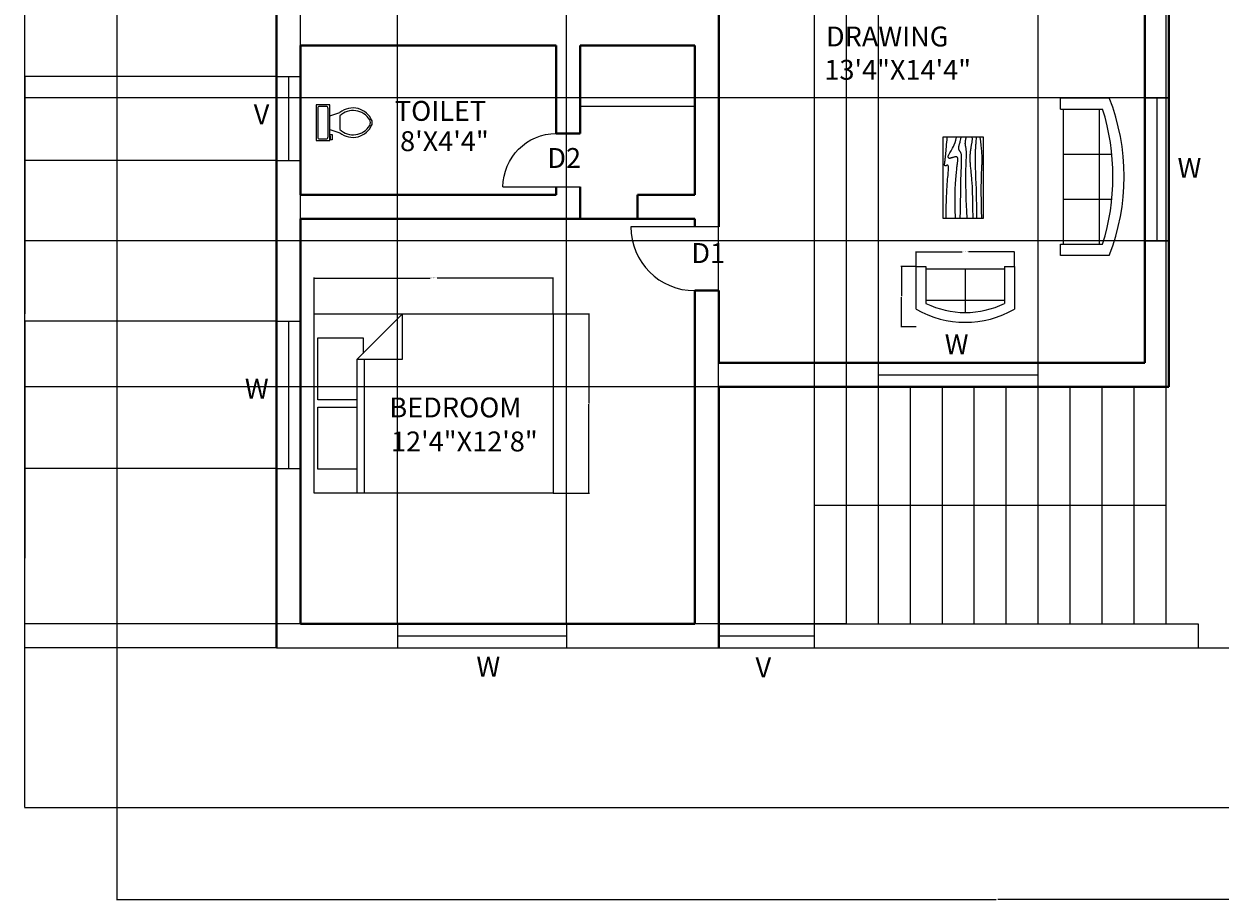
# Model space of a CAD drawing. Units: feet. Extents: x 2032 to 2763, y 1402 to 2145.
# Tile 1 of 6: x 2032 to 2482, y 1402 to 1731. Entities that reach past the tile are written whole.
import ezdxf

# ---------------------------------------------------------------- set-up
doc = ezdxf.new("R2010")
doc.units = ezdxf.units.FT
for name, color, linetype, lineweight in [('A-ANNO-DIMS', 2, 'Continuous', 18), ('A-ANNO-TEXT', 7, 'Continuous', 18), ('A-AREA-IDEN', 7, 'Continuous', 25), ('A-DOOR', 3, 'Continuous', 25), ('A-FLOR', 7, 'Continuous', 25), ('A-FLOR-CASE', 8, 'Continuous', 18), ('A-FLOR-FIXT', 8, 'Continuous', 18), ('A-FLOR-STRS', 7, 'Continuous', 18), ('A-FURN', 8, 'Continuous', 18), ('A-GLAZ', 4, 'Continuous', 18), ('A-WALL', 7, 'Continuous', 40), ('C-PROP', 8, 'Continuous', 25)]:
    doc.layers.add(name, color=color, linetype=linetype, lineweight=lineweight)
doc.styles.get("Standard").update_dxf_attribs({"font": 'arial.ttf'})
doc.dimstyles.get("Standard").update_dxf_attribs({"dimtxt": 0.18, "dimasz": 0.18, "dimexe": 0.18, "dimexo": 0.0625, "dimgap": 0.09, "dimtad": 0, "dimtih": 1, "dimtoh": 1, "dimdec": 4, "dimzin": 0, "dimdsep": 46, "dimtxsty": 'Standard', "dimcen": 0.09, "dimadec": 0, "dimazin": 0, "dimtfac": 1, "dimtdec": 4, "dimtofl": 0, "dimtmove": 0, "dimatfit": 3, "dimfxl": 1, "dimtolj": 1, "dimtzin": 0, "dimarcsym": 0})

# ---------------------------------------------------------------- blocks, each defined once
blk = doc.blocks.new('Bed - Queen')
for p, q in [((0, -80.00003), (0, 0)), ((0, 0), (59.99999, 0)), ((59.99999, 0), (59.99999, -80.00003)), ((7.99999, -1.2), (28.79998, -1.2)), ((7.99999, -14.4), (7.99999, -1.2)), ((28.79998, -1.2), (28.79998, -14.4)), ((31.19999, -1.2), (51.99999, -1.2)), ((31.19999, -14.4), (31.19999, -1.2)), ((51.99999, -1.2), (51.99999, -16.4)), ((0, -14.4), (44.8, -14.4)), ((59.99999, -29.6), (44.8, -14.4)), ((44.8, -14.4), (44.8, -29.6)), ((44.8, -16.8), (0, -16.8)), ((51.99999, -16.4), (46.79936, -16.4)), ((44.8, -29.6), (59.99999, -29.6)), ((59.99999, -80.00003), (0, -80.00003))]:
    blk.add_line(p, q)
blk = doc.blocks.new('Sofa - Roundback 7 ft.')
for p, q in [((-36.000027, -34), (-36.000027, -11.4696)), ((-12.00002, -32.4421), (-12.00003, -6.5971)), ((11.99997, -32.4421), (11.99998, -6.5971)), ((35.99998, -34), (35.99998, -11.4696)), ((-35.999844, -13.3819), (35.9998, -13.3819)), ((-36.000027, -32.4421), (35.99998, -32.4421))]:
    blk.add_line(p, q)
for points in [[(-36.000027, -34), (-42.000027, -34), (-42.000027, -8)], [(41.99998, -8), (41.99998, -34), (35.99998, -34)]]:
    blk.add_lwpolyline(points)
for centre, radius, start, end in [((0, -114.25), 114.25, 68.43141, 111.5686), ((-0.00001, -127.1968), 121.1968, 72.72033, 107.2797)]:
    blk.add_arc(centre, radius, start, end)
blk = doc.blocks.new('Sofa - Roundback Loveseat 5 ft.')
for p, q in [((0, -32.44198), (0, -5.99998)), ((-24, -33.99998), (-24, -11.46958)), ((-23.9998, -13.38178), (23.99986, -13.38178)), ((24.00004, -33.99998), (24.00004, -11.46958)), ((-24, -32.44198), (24.00004, -32.44198))]:
    blk.add_line(p, q)
for points in [[(-24, -33.99998), (-30, -33.99998), (-30, -7.99998)], [(30.00004, -7.99998), (30.00004, -33.99998), (24.00004, -33.99998)]]:
    blk.add_lwpolyline(points)
for centre, radius, start, end in [((0, -60.24998), 60.24998, 60.13715, 119.8628), ((0, -61.38438), 55.38444, 64.32083, 115.6792)]:
    blk.add_arc(centre, radius, start, end)
blk = doc.blocks.new('Table - Rectangular Woodgrain 60 x 30 in.')
for p, q in [((0, 0), (0, -30)), ((60, 0), (0, 0)), ((60, -30), (60, 0)), ((0, -30), (60, -30))]:
    blk.add_line(p, q)
for points in [[(0, -2.4), (4.8155, -2.418), (9.0302, -2.4688), (12.709, -2.5477), (15.9167, -2.65), (18.7181, -2.7711), (21.1781, -2.9063), (23.3616, -3.0508), (25.3333, -3.2), (27.1477, -3.3495), (28.8172, -3.4958), (30.3437, -3.636), (31.7291, -3.7667), (32.9756, -3.8849), (34.0849, -3.9875), (35.059, -4.0714), (35.9, -4.1334), (36.6114, -4.1711), (37.2041, -4.1854), (37.6906, -4.1779), (38.0833, -4.15), (38.3948, -4.1034), (38.6375, -4.0396), (38.8239, -3.9602), (38.9666, -3.8667), (39.0764, -3.7608), (39.1573, -3.6448), (39.2116, -3.521), (39.2416, -3.3917), (39.2498, -3.2593), (39.2385, -3.1261), (39.21, -2.9944), (39.1666, -2.8667), (39.111, -2.7447), (39.0468, -2.6281), (38.978, -2.5163), (38.9083, -2.4083), (38.8418, -2.3035), (38.7823, -2.201), (38.7337, -2.1001), (38.7, -2), (38.6844, -1.9003), (38.6875, -1.8021), (38.7094, -1.707), (38.75, -1.6167), (38.8094, -1.5326), (38.8875, -1.4563), (38.9844, -1.3893), (39.1, -1.3333), (39.2351, -1.2896), (39.3937, -1.2583), (39.5804, -1.2396), (39.8, -1.2333), (40.057, -1.2396), (40.3562, -1.2583), (40.7023, -1.2896), (41.1, -1.3333), (41.5547, -1.3895), (42.0755, -1.4573), (42.6721, -1.5361), (43.3542, -1.625), (44.1316, -1.7233), (45.014, -1.8302), (46.0114, -1.9449), (47.1333, -2.0667), (48.3862, -2.1947), (49.7625, -2.3281), (51.2513, -2.4663), (52.8416, -2.6083), (54.5226, -2.7535), (56.2833, -2.9011), (58.1127, -3.0501), (60, -3.2)], [(0, -9.2), (6.5759, -9.0858), (11.9385, -9.0365), (16.2527, -9.0418), (19.6833, -9.0917), (22.3952, -9.1759), (24.5531, -9.2844), (26.322, -9.4069), (27.8666, -9.5333), (29.3241, -9.6553), (30.7203, -9.7719), (32.0532, -9.8837), (33.3208, -9.9917), (34.5213, -10.0965), (35.6526, -10.199), (36.7128, -10.2999), (37.7, -10.4), (38.6129, -10.4996), (39.4531, -10.5969), (40.223, -10.6895), (40.925, -10.775), (41.5613, -10.8512), (42.1344, -10.9156), (42.6465, -10.966), (43.1, -11), (43.4976, -11.0158), (43.8437, -11.0136), (44.143, -10.9942), (44.4, -10.9583), (44.6195, -10.9069), (44.8062, -10.8406), (44.9648, -10.7603), (45.1, -10.6667), (45.2155, -10.5598), (45.3114, -10.4365), (45.3871, -10.2929), (45.4416, -10.125), (45.4743, -9.929), (45.4844, -9.7011), (45.4709, -9.4371), (45.4333, -9.1333), (45.3716, -8.7883), (45.2896, -8.4104), (45.1919, -8.0107), (45.0833, -7.6), (44.9685, -7.1893), (44.8521, -6.7896), (44.7388, -6.4117), (44.6333, -6.0667), (44.54, -5.7628), (44.4614, -5.4979), (44.4001, -5.2675), (44.3583, -5.0667), (44.3384, -4.8909), (44.3427, -4.7354), (44.3736, -4.5956), (44.4333, -4.4667), (44.5236, -4.3453), (44.6427, -4.2333), (44.7884, -4.1339), (44.9583, -4.05), (45.1501, -3.9849), (45.3614, -3.9417), (45.59, -3.9234), (45.8333, -3.9333), (46.0915, -3.9749), (46.3734, -4.0531), (46.6906, -4.1736), (47.0542, -4.3417), (47.4756, -4.5629), (47.9661, -4.8427), (48.5372, -5.1866), (49.2, -5.6), (49.9676, -6.0844), (50.8594, -6.625), (51.8965, -7.2031), (53.1, -7.8), (54.491, -8.3969), (56.0906, -8.975), (57.9199, -9.5156), (60, -10)], [(0, -12.8), (5.1847, -12.9322), (9.6213, -13.0323), (13.3963, -13.1059), (16.5958, -13.1583), (19.3063, -13.1952), (21.614, -13.2219), (23.6054, -13.2439), (25.3666, -13.2667), (26.9728, -13.2947), (28.4531, -13.3281), (29.8256, -13.3663), (31.1083, -13.4083), (32.3191, -13.4535), (33.476, -13.501), (34.597, -13.5501), (35.7, -13.6), (36.7984, -13.6497), (37.8875, -13.6979), (38.9578, -13.743), (40, -13.7833), (41.0047, -13.8174), (41.9625, -13.8438), (42.864, -13.8607), (43.7, -13.8667), (44.4631, -13.8604), (45.1552, -13.8417), (45.7801, -13.8104), (46.3416, -13.7667), (46.8439, -13.7104), (47.2906, -13.6417), (47.6858, -13.5604), (48.0333, -13.4667), (48.3375, -13.3608), (48.6042, -13.2448), (48.8396, -13.121), (49.05, -12.9917), (49.2417, -12.8593), (49.4208, -12.7261), (49.5937, -12.5944), (49.7667, -12.4667), (49.9452, -12.3451), (50.1323, -12.2313), (50.3303, -12.1268), (50.5416, -12.0333), (50.7686, -11.9524), (51.0135, -11.8854), (51.2788, -11.8341), (51.5666, -11.8), (51.8785, -11.7843), (52.2116, -11.7865), (52.562, -11.8059), (52.926, -11.8417), (53.2998, -11.8931), (53.6795, -11.9594), (54.0614, -12.0397), (54.4416, -12.1333), (54.8223, -12.2401), (55.2293, -12.3625), (55.6942, -12.5037), (56.2489, -12.6667), (56.9251, -12.8547), (57.7545, -13.0708), (58.7689, -13.3182), (60, -13.6)], [(0, -18), (5.124, -17.7273), (9.6609, -17.5057), (13.6705, -17.3303), (17.2125, -17.1958), (20.3467, -17.0973), (23.1328, -17.0297), (25.6307, -16.9878), (27.9, -16.9667), (29.9928, -16.9617), (31.9302, -16.9703), (33.7254, -16.9907), (35.3917, -17.0208), (36.9423, -17.0588), (38.3906, -17.1026), (39.7499, -17.1503), (41.0333, -17.2), (42.2519, -17.2496), (43.4073, -17.2969), (44.4986, -17.3395), (45.525, -17.375), (46.4858, -17.4012), (47.3802, -17.4156), (48.2074, -17.416), (48.9667, -17.4), (49.6583, -17.3662), (50.2872, -17.3167), (50.8595, -17.2547), (51.3812, -17.1833), (51.8584, -17.1057), (52.2971, -17.025), (52.7034, -16.9443), (53.0833, -16.8667), (53.443, -16.7951), (53.789, -16.7313), (54.128, -16.6768), (54.4666, -16.6334), (54.8115, -16.6024), (55.1693, -16.5854), (55.5465, -16.5841), (55.95, -16.6), (56.3828, -16.6337), (56.8346, -16.6823), (57.2915, -16.7418), (57.7396, -16.8084), (58.165, -16.878), (58.5539, -16.9469), (58.8924, -17.0111), (59.1666, -17.0667), (59.3679, -17.1107), (59.5078, -17.1438), (59.6032, -17.1675), (59.6708, -17.1833), (59.7275, -17.193), (59.7901, -17.1979), (59.8753, -17.1998), (60, -17.2)], [(0, -22.4), (8.0098, -22.2501), (14.4094, -22.1011), (19.4168, -21.9535), (23.25, -21.8083), (26.1269, -21.6663), (28.2656, -21.5281), (29.884, -21.3947), (31.2, -21.2667), (32.3967, -21.1448), (33.5172, -21.0292), (34.5697, -20.9198), (35.5625, -20.8167), (36.5037, -20.7198), (37.4015, -20.6292), (38.2642, -20.5448), (39.1, -20.4667), (39.9164, -20.3951), (40.7187, -20.3313), (41.5117, -20.2768), (42.3, -20.2333), (43.0883, -20.2024), (43.8812, -20.1854), (44.6836, -20.1841), (45.5, -20.2), (46.3328, -20.234), (47.1747, -20.2844), (48.0163, -20.3488), (48.8479, -20.425), (49.66, -20.5106), (50.4429, -20.6031), (51.1872, -20.7004), (51.8833, -20.8), (52.5246, -20.8999), (53.1166, -20.9995), (53.6681, -21.0983), (54.1875, -21.1958), (54.6834, -21.2919), (55.1646, -21.3859), (55.6394, -21.4777), (56.1167, -21.5667), (56.6028, -21.6515), (57.0961, -21.7266), (57.5929, -21.7852), (58.0896, -21.8208), (58.5823, -21.8268), (59.0674, -21.7964), (59.5412, -21.723), (60, -21.6)], [(0, -25.2), (8.6355, -25.0504), (15.7026, -24.9031), (21.4049, -24.7606), (25.9458, -24.625), (29.529, -24.4988), (32.3578, -24.3844), (34.6359, -24.284), (36.5667, -24.2), (38.3213, -24.1341), (39.9417, -24.0854), (41.437, -24.0523), (42.8167, -24.0333), (44.0901, -24.0268), (45.2667, -24.0313), (46.3557, -24.0451), (47.3667, -24.0667), (48.309, -24.0947), (49.1928, -24.1287), (50.0284, -24.168), (50.826, -24.2125), (51.5959, -24.2617), (52.3483, -24.3151), (53.0935, -24.3725), (53.8417, -24.4334), (54.6009, -24.497), (55.3699, -24.561), (56.1454, -24.6226), (56.9239, -24.6792), (57.7021, -24.7279), (58.4764, -24.7662), (59.2435, -24.7911), (60, -24.8)], [(0, -28.8), (5.6867, -28.6681), (10.45, -28.5698), (14.407, -28.5012), (17.675, -28.4584), (20.3711, -28.4374), (22.6125, -28.4344), (24.5164, -28.4455), (26.2, -28.4667), (27.762, -28.4947), (29.2276, -28.5281), (30.6033, -28.5663), (31.8958, -28.6084), (33.1118, -28.6535), (34.2578, -28.7011), (35.3405, -28.7501), (36.3666, -28.8), (37.3443, -28.8497), (38.288, -28.8974), (39.2137, -28.9412), (40.1375, -28.9792), (41.0753, -29.0093), (42.0432, -29.0297), (43.0572, -29.0384), (44.1333, -29.0333), (45.2936, -29.0114), (46.5843, -28.9641), (48.0579, -28.8816), (49.7666, -28.7542), (51.7629, -28.5721), (54.0989, -28.3255), (56.8272, -28.0048), (60, -27.6)]]:
    blk.add_lwpolyline(points)
blk = doc.blocks.new('Toilet - top')
for p, q in [((9.5, -6), (9.5, -2)), ((-10, -8.5), (-8, -8.5)), ((-10, -9.5), (-10, -8.5)), ((-7, -9.5), (-10, -9.5)), ((-8, -8.5), (-8, -8)), ((-7, -8), (-7, -9.5)), ((-4, -8), (-6, -14)), ((4, -14), (-4, -14)), ((4, -8), (6, -14))]:
    blk.add_line(p, q)
blk.add_lwpolyline([(10.5, -8), (10.5, 0), (-10.5, 0), (-10.5, -8)], close=True)
for points in [[(-9.5, -2), (-9.5, -6)], [(8.5, -1), (-8.5, -1)], [(-8.5, -7), (8.5, -7)]]:
    blk.add_lwpolyline(points)
for centre, radius, start, end in [((-8.62, -1.88), 0.884, 81.8699, 188.1301), ((-8.62, -6.12), 0.884, 171.8699, 278.1301), ((8.62, -1.88), 0.884, 351.8699, 98.1301), ((8.62, -6.12), 0.884, 261.8699, 8.1301), ((3.52, -21.58), 12.17, 141.46911, 247.97143), ((4.2, -21.82), 11.33, 136.36773, 238.94682), ((-3.52, -21.58), 12.17, 292.02843, 38.53071), ((-4.2, -21.82), 11.33, 301.05301, 43.63209), ((0, -27.88), 4, 245.73182, 294.26817), ((0, -29), 4, 254.86053, 285.13947)]:
    blk.add_arc(centre, radius, start, end)
blk = doc.blocks.new('DOOR-SWING-20')
blk.add_line((0, 20), (29, 20))
blk.add_arc((20, 20), 20, 180, 270)
blk = doc.blocks.new('*D15')
at = {"layer": 'A-ANNO-DIMS', "color": 0, "lineweight": -2, "transparency": 16777216}
for p, q in [((2141.39, 1621.99), (2141.39, 1635.57)), ((2141.57, 1635.39), (2184.95, 1635.39)), ((2230.94, 1635.39), (2187.56, 1635.39)), ((2231.12, 1621.99), (2231.12, 1635.57))]:
    blk.add_line(p, q, dxfattribs=at)
at = {"layer": 'A-ANNO-DIMS', "color": 0, "transparency": 16777216}
for points in [[(2141.57, 1635.42), (2141.57, 1635.36), (2141.39, 1635.39)], [(2230.94, 1635.42), (2230.94, 1635.36), (2231.12, 1635.39)]]:
    blk.add_solid(points, dxfattribs=at)
at = {"layer": 'Defpoints', "color": 0, "transparency": 16777216}
for p in [(2141.39, 1635.39), (2141.39, 1621.93), (2231.12, 1621.93)]:
    blk.add_point(p, dxfattribs=at)
at = {"layer": 'A-ANNO-DIMS', "color": 0, "transparency": 16777216, "insert": (2186.26, 1635.39), "char_height": 0.18, "attachment_point": 5}
blk.add_mtext('\\A1;QUEEN BED 90 TYP.', dxfattribs=at)
blk = doc.blocks.new('*D16')
at = {"layer": 'A-ANNO-DIMS', "color": 0, "lineweight": -2, "transparency": 16777216}
for p, q in [((2231.18, 1621.93), (2244.76, 1621.93)), ((2244.58, 1621.75), (2244.58, 1588.47)), ((2244.58, 1554.82), (2244.58, 1588.1)), ((2231.18, 1554.64), (2244.76, 1554.64))]:
    blk.add_line(p, q, dxfattribs=at)
at = {"layer": 'A-ANNO-DIMS', "color": 0, "transparency": 16777216}
for points in [[(2244.55, 1621.75), (2244.61, 1621.75), (2244.58, 1621.93)], [(2244.55, 1554.82), (2244.61, 1554.82), (2244.58, 1554.64)]]:
    blk.add_solid(points, dxfattribs=at)
at = {"layer": 'Defpoints', "color": 0, "transparency": 16777216}
for p in [(2231.12, 1621.93), (2244.58, 1621.93), (2231.12, 1554.64)]:
    blk.add_point(p, dxfattribs=at)
at = {"layer": 'A-ANNO-DIMS', "color": 0, "transparency": 16777216, "insert": (2244.58, 1588.28), "char_height": 0.18, "attachment_point": 5}
blk.add_mtext('\\A1;67 TYP.', dxfattribs=at)
blk = doc.blocks.new('*D19')
at = {"layer": 'A-ANNO-DIMS', "color": 0, "lineweight": -2, "transparency": 16777216}
for p, q in [((2367.48, 1639.73), (2367.48, 1645.38)), ((2367.66, 1645.2), (2384.69, 1645.2)), ((2404.17, 1645.2), (2387.14, 1645.2)), ((2404.35, 1639.73), (2404.35, 1645.38))]:
    blk.add_line(p, q, dxfattribs=at)
at = {"layer": 'A-ANNO-DIMS', "color": 0, "transparency": 16777216}
for points in [[(2367.66, 1645.23), (2367.66, 1645.17), (2367.48, 1645.2)], [(2404.17, 1645.23), (2404.17, 1645.17), (2404.35, 1645.2)]]:
    blk.add_solid(points, dxfattribs=at)
at = {"layer": 'Defpoints', "color": 0, "transparency": 16777216}
for p in [(2367.48, 1645.2), (2367.48, 1639.67), (2404.35, 1639.67)]:
    blk.add_point(p, dxfattribs=at)
at = {"layer": 'A-ANNO-DIMS', "color": 0, "transparency": 16777216, "insert": (2385.91, 1645.2), "char_height": 0.18, "attachment_point": 5}
blk.add_mtext('\\A1;LOVESEAT 37 TYP.', dxfattribs=at)
blk = doc.blocks.new('*D20')
at = {"layer": 'A-ANNO-DIMS', "color": 0, "lineweight": -2, "transparency": 16777216}
for p, q in [((2367.42, 1639.67), (2361.77, 1639.67)), ((2361.95, 1639.49), (2361.95, 1628.58)), ((2361.95, 1617.31), (2361.95, 1628.22)), ((2367.42, 1617.13), (2361.77, 1617.13))]:
    blk.add_line(p, q, dxfattribs=at)
at = {"layer": 'A-ANNO-DIMS', "color": 0, "transparency": 16777216}
for points in [[(2361.92, 1639.49), (2361.98, 1639.49), (2361.95, 1639.67)], [(2361.92, 1617.31), (2361.98, 1617.31), (2361.95, 1617.13)]]:
    blk.add_solid(points, dxfattribs=at)
at = {"layer": 'Defpoints', "color": 0, "transparency": 16777216}
for p in [(2367.48, 1639.67), (2361.95, 1617.13), (2367.48, 1617.13)]:
    blk.add_point(p, dxfattribs=at)
at = {"layer": 'A-ANNO-DIMS', "color": 0, "transparency": 16777216, "insert": (2361.95, 1628.4), "char_height": 0.18, "attachment_point": 5}
blk.add_mtext('\\A1;23 TYP.', dxfattribs=at)
blk = doc.blocks.new('*D33')
at = {"layer": 'A-ANNO-DIMS', "color": 0, "lineweight": -2, "transparency": 16777216}
for p, q in [((2067.31, 1436.55), (2067.31, 1401.93)), ((2728.31, 1436.55), (2728.31, 1401.93)), ((2067.49, 1402.11), (2397.54, 1402.11)), ((2728.13, 1402.11), (2398.09, 1402.11))]:
    blk.add_line(p, q, dxfattribs=at)
at = {"layer": 'A-ANNO-DIMS', "color": 0, "transparency": 16777216}
for points in [[(2067.49, 1402.14), (2067.49, 1402.08), (2067.31, 1402.11)], [(2728.13, 1402.14), (2728.13, 1402.08), (2728.31, 1402.11)]]:
    blk.add_solid(points, dxfattribs=at)
at = {"layer": 'Defpoints', "color": 0, "transparency": 16777216}
for p in [(2067.31, 1436.61), (2728.31, 1436.61), (2728.31, 1402.11)]:
    blk.add_point(p, dxfattribs=at)
at = {"layer": 'A-ANNO-DIMS', "color": 0, "transparency": 16777216, "insert": (2397.81, 1402.11), "char_height": 0.18, "attachment_point": 5}
blk.add_mtext('\\A1;661', dxfattribs=at)
blk = doc.blocks.new('*D34')
at = {"layer": 'A-ANNO-DIMS', "color": 0, "lineweight": -2, "transparency": 16777216}
for p, q in [((2067.25, 2110.61), (2032.63, 2110.61)), ((2032.81, 2110.43), (2032.81, 1773.79)), ((2032.81, 1436.79), (2032.81, 1773.43)), ((2067.25, 1436.61), (2032.63, 1436.61))]:
    blk.add_line(p, q, dxfattribs=at)
at = {"layer": 'A-ANNO-DIMS', "color": 0, "transparency": 16777216}
for points in [[(2032.78, 2110.43), (2032.84, 2110.43), (2032.81, 2110.61)], [(2032.78, 1436.79), (2032.84, 1436.79), (2032.81, 1436.61)]]:
    blk.add_solid(points, dxfattribs=at)
at = {"layer": 'Defpoints', "color": 0, "transparency": 16777216}
for p in [(2032.81, 2110.61), (2067.31, 2110.61), (2067.31, 1436.61)]:
    blk.add_point(p, dxfattribs=at)
at = {"layer": 'A-ANNO-DIMS', "color": 0, "transparency": 16777216, "insert": (2032.81, 1773.61), "char_height": 0.18, "attachment_point": 5}
blk.add_mtext('\\A1;674', dxfattribs=at)
blk = doc.blocks.new('*D49')
at = {"layer": 'A-ANNO-DIMS', "color": 0, "lineweight": -2, "transparency": 16777216}
for p, q in [((2127.25, 1563.86), (2032.63, 1563.86)), ((2032.81, 1563.68), (2032.81, 1530.42)), ((2032.81, 1496.79), (2032.81, 1530.05)), ((2127.25, 1496.61), (2032.63, 1496.61))]:
    blk.add_line(p, q, dxfattribs=at)
at = {"layer": 'A-ANNO-DIMS', "color": 0, "transparency": 16777216}
for points in [[(2032.78, 1563.68), (2032.84, 1563.68), (2032.81, 1563.86)], [(2032.78, 1496.79), (2032.84, 1496.79), (2032.81, 1496.61)]]:
    blk.add_solid(points, dxfattribs=at)
at = {"layer": 'Defpoints', "color": 0, "transparency": 16777216}
for p in [(2032.81, 1563.86), (2127.31, 1563.86), (2127.31, 1496.61)]:
    blk.add_point(p, dxfattribs=at)
at = {"layer": 'A-ANNO-DIMS', "color": 0, "transparency": 16777216, "insert": (2032.81, 1530.23), "char_height": 0.18, "attachment_point": 5}
blk.add_mtext('\\A1;67.24', dxfattribs=at)
blk = doc.blocks.new('*D50')
at = {"layer": 'A-ANNO-DIMS', "color": 0, "lineweight": -2, "transparency": 16777216}
for p, q in [((2127.25, 1619.16), (2032.63, 1619.16)), ((2032.81, 1618.98), (2032.81, 1591.69)), ((2032.81, 1564.04), (2032.81, 1591.33)), ((2127.25, 1563.86), (2032.63, 1563.86))]:
    blk.add_line(p, q, dxfattribs=at)
at = {"layer": 'A-ANNO-DIMS', "color": 0, "transparency": 16777216}
for points in [[(2032.78, 1618.98), (2032.84, 1618.98), (2032.81, 1619.16)], [(2032.78, 1564.04), (2032.84, 1564.04), (2032.81, 1563.86)]]:
    blk.add_solid(points, dxfattribs=at)
at = {"layer": 'Defpoints', "color": 0, "transparency": 16777216}
for p in [(2032.81, 1619.16), (2127.31, 1619.16), (2127.31, 1563.86)]:
    blk.add_point(p, dxfattribs=at)
at = {"layer": 'A-ANNO-DIMS', "color": 0, "transparency": 16777216, "insert": (2032.81, 1591.51), "char_height": 0.18, "attachment_point": 5}
blk.add_mtext('\\A1;55.31', dxfattribs=at)
blk = doc.blocks.new('*D51')
at = {"layer": 'A-ANNO-DIMS', "color": 0, "lineweight": -2, "transparency": 16777216}
for p, q in [((2127.25, 1679.46), (2032.63, 1679.46)), ((2032.81, 1679.28), (2032.81, 1649.49)), ((2032.81, 1619.34), (2032.81, 1649.13)), ((2127.25, 1619.16), (2032.63, 1619.16))]:
    blk.add_line(p, q, dxfattribs=at)
at = {"layer": 'A-ANNO-DIMS', "color": 0, "transparency": 16777216}
for points in [[(2032.78, 1679.28), (2032.84, 1679.28), (2032.81, 1679.46)], [(2032.78, 1619.34), (2032.84, 1619.34), (2032.81, 1619.16)]]:
    blk.add_solid(points, dxfattribs=at)
at = {"layer": 'Defpoints', "color": 0, "transparency": 16777216}
for p in [(2032.81, 1679.46), (2127.31, 1679.46), (2127.31, 1619.16)]:
    blk.add_point(p, dxfattribs=at)
at = {"layer": 'A-ANNO-DIMS', "color": 0, "transparency": 16777216, "insert": (2032.81, 1649.31), "char_height": 0.18, "attachment_point": 5}
blk.add_mtext('\\A1;60.3', dxfattribs=at)
blk = doc.blocks.new('*D52')
at = {"layer": 'A-ANNO-DIMS', "color": 0, "lineweight": -2, "transparency": 16777216}
for p, q in [((2127.25, 1711), (2032.63, 1711)), ((2032.81, 1710.82), (2032.81, 1695.41)), ((2032.81, 1679.64), (2032.81, 1695.05)), ((2127.25, 1679.46), (2032.63, 1679.46))]:
    blk.add_line(p, q, dxfattribs=at)
at = {"layer": 'A-ANNO-DIMS', "color": 0, "transparency": 16777216}
for points in [[(2032.78, 1710.82), (2032.84, 1710.82), (2032.81, 1711)], [(2032.78, 1679.64), (2032.84, 1679.64), (2032.81, 1679.46)]]:
    blk.add_solid(points, dxfattribs=at)
at = {"layer": 'Defpoints', "color": 0, "transparency": 16777216}
for p in [(2032.81, 1711), (2127.31, 1711), (2127.31, 1679.46)]:
    blk.add_point(p, dxfattribs=at)
at = {"layer": 'A-ANNO-DIMS', "color": 0, "transparency": 16777216, "insert": (2032.81, 1695.23), "char_height": 0.18, "attachment_point": 5}
blk.add_mtext('\\A1;31.534', dxfattribs=at)
blk = doc.blocks.new('*D53')
at = {"layer": 'A-ANNO-DIMS', "color": 0, "lineweight": -2, "transparency": 16777216}
for p, q in [((2127.25, 1765.5), (2032.63, 1765.5)), ((2032.81, 1765.32), (2032.81, 1738.43)), ((2032.81, 1711.18), (2032.81, 1738.07)), ((2127.25, 1711), (2032.63, 1711))]:
    blk.add_line(p, q, dxfattribs=at)
at = {"layer": 'A-ANNO-DIMS', "color": 0, "transparency": 16777216}
for points in [[(2032.78, 1765.32), (2032.84, 1765.32), (2032.81, 1765.5)], [(2032.78, 1711.18), (2032.84, 1711.18), (2032.81, 1711)]]:
    blk.add_solid(points, dxfattribs=at)
at = {"layer": 'Defpoints', "color": 0, "transparency": 16777216}
for p in [(2032.81, 1765.5), (2127.31, 1765.5), (2127.31, 1711)]:
    blk.add_point(p, dxfattribs=at)
at = {"layer": 'A-ANNO-DIMS', "color": 0, "transparency": 16777216, "insert": (2032.81, 1738.25), "char_height": 0.18, "attachment_point": 5}
blk.add_mtext('\\A1;54.5', dxfattribs=at)
blk = doc.blocks.new('*D67')
at = {"layer": 'A-ANNO-DIMS', "color": 0, "lineweight": -2, "transparency": 16777216}
for p, q in [((2329.31, 1594.68), (2329.31, 2145.29)), ((2329.49, 2145.11), (2395.03, 2145.11)), ((2461.13, 2145.11), (2395.59, 2145.11)), ((2461.31, 1594.68), (2461.31, 2145.29))]:
    blk.add_line(p, q, dxfattribs=at)
at = {"layer": 'A-ANNO-DIMS', "color": 0, "transparency": 16777216}
for points in [[(2329.49, 2145.14), (2329.49, 2145.08), (2329.31, 2145.11)], [(2461.13, 2145.14), (2461.13, 2145.08), (2461.31, 2145.11)]]:
    blk.add_solid(points, dxfattribs=at)
at = {"layer": 'Defpoints', "color": 0, "transparency": 16777216}
for p in [(2461.31, 2145.11), (2329.31, 1594.61), (2461.31, 1594.61)]:
    blk.add_point(p, dxfattribs=at)
at = {"layer": 'A-ANNO-DIMS', "color": 0, "transparency": 16777216, "insert": (2395.31, 2145.11), "char_height": 0.18, "attachment_point": 5}
blk.add_mtext('\\A1;132', dxfattribs=at)
blk = doc.blocks.new('*D68')
at = {"layer": 'A-ANNO-DIMS', "color": 0, "lineweight": -2, "transparency": 16777216}
for p, q in [((2341.25, 1594.61), (2032.63, 1594.61)), ((2032.81, 1594.43), (2032.81, 1550.29)), ((2032.81, 1505.79), (2032.81, 1549.93)), ((2341.25, 1505.61), (2032.63, 1505.61))]:
    blk.add_line(p, q, dxfattribs=at)
at = {"layer": 'A-ANNO-DIMS', "color": 0, "transparency": 16777216}
for points in [[(2032.78, 1594.43), (2032.84, 1594.43), (2032.81, 1594.61)], [(2032.78, 1505.79), (2032.84, 1505.79), (2032.81, 1505.61)]]:
    blk.add_solid(points, dxfattribs=at)
at = {"layer": 'Defpoints', "color": 0, "transparency": 16777216}
for p in [(2032.81, 1594.61), (2341.31, 1594.61), (2341.31, 1505.61)]:
    blk.add_point(p, dxfattribs=at)
at = {"layer": 'A-ANNO-DIMS', "color": 0, "transparency": 16777216, "insert": (2032.81, 1550.11), "char_height": 0.18, "attachment_point": 5}
blk.add_mtext('\\A1;89', dxfattribs=at)
blk = doc.blocks.new('*D69')
at = {"layer": 'A-ANNO-DIMS', "color": 0, "lineweight": -2, "transparency": 16777216}
for p, q in [((2341.31, 1505.68), (2341.31, 2145.29)), ((2341.49, 2145.11), (2347.1, 2145.11)), ((2353.13, 2145.11), (2347.52, 2145.11)), ((2353.31, 1505.68), (2353.31, 2145.29))]:
    blk.add_line(p, q, dxfattribs=at)
at = {"layer": 'A-ANNO-DIMS', "color": 0, "transparency": 16777216}
for points in [[(2341.49, 2145.14), (2341.49, 2145.08), (2341.31, 2145.11)], [(2353.13, 2145.14), (2353.13, 2145.08), (2353.31, 2145.11)]]:
    blk.add_solid(points, dxfattribs=at)
at = {"layer": 'Defpoints', "color": 0, "transparency": 16777216}
for p in [(2353.31, 2145.11), (2341.31, 1505.61), (2353.31, 1505.61)]:
    blk.add_point(p, dxfattribs=at)
at = {"layer": 'A-ANNO-DIMS', "color": 0, "transparency": 16777216, "insert": (2347.31, 2145.11), "char_height": 0.18, "attachment_point": 5}
blk.add_mtext('\\A1;12', dxfattribs=at)
blk = doc.blocks.new('*D70')
at = {"layer": 'A-ANNO-DIMS', "color": 0, "lineweight": -2, "transparency": 16777216}
for p, q in [((2136.31, 1505.68), (2136.31, 2145.29)), ((2136.49, 2145.11), (2154.19, 2145.11)), ((2172.54, 2145.11), (2154.84, 2145.11)), ((2172.72, 1505.68), (2172.72, 2145.29))]:
    blk.add_line(p, q, dxfattribs=at)
at = {"layer": 'A-ANNO-DIMS', "color": 0, "transparency": 16777216}
for points in [[(2136.49, 2145.14), (2136.49, 2145.08), (2136.31, 2145.11)], [(2172.54, 2145.14), (2172.54, 2145.08), (2172.72, 2145.11)]]:
    blk.add_solid(points, dxfattribs=at)
at = {"layer": 'Defpoints', "color": 0, "transparency": 16777216}
for p in [(2172.72, 2145.11), (2136.31, 1505.61), (2172.72, 1505.61)]:
    blk.add_point(p, dxfattribs=at)
at = {"layer": 'A-ANNO-DIMS', "color": 0, "transparency": 16777216, "insert": (2154.51, 2145.11), "char_height": 0.18, "attachment_point": 5}
blk.add_mtext('\\A1;36.4', dxfattribs=at)
blk = doc.blocks.new('*D71')
at = {"layer": 'A-ANNO-DIMS', "color": 0, "lineweight": -2, "transparency": 16777216}
for p, q in [((2172.72, 1505.68), (2172.72, 2145.29)), ((2172.9, 2145.11), (2204.05, 2145.11)), ((2236, 2145.11), (2204.84, 2145.11)), ((2236.18, 1505.68), (2236.18, 2145.29))]:
    blk.add_line(p, q, dxfattribs=at)
at = {"layer": 'A-ANNO-DIMS', "color": 0, "transparency": 16777216}
for points in [[(2172.9, 2145.14), (2172.9, 2145.08), (2172.72, 2145.11)], [(2236, 2145.14), (2236, 2145.08), (2236.18, 2145.11)]]:
    blk.add_solid(points, dxfattribs=at)
at = {"layer": 'Defpoints', "color": 0, "transparency": 16777216}
for p in [(2236.18, 2145.11), (2172.72, 1505.61), (2236.18, 1505.61)]:
    blk.add_point(p, dxfattribs=at)
at = {"layer": 'A-ANNO-DIMS', "color": 0, "transparency": 16777216, "insert": (2204.45, 2145.11), "char_height": 0.18, "attachment_point": 5}
blk.add_mtext('\\A1;63.46', dxfattribs=at)
blk = doc.blocks.new('*D72')
at = {"layer": 'A-ANNO-DIMS', "color": 0, "lineweight": -2, "transparency": 16777216}
for p, q in [((2293.31, 1505.68), (2293.31, 2145.29)), ((2293.49, 2145.11), (2311.09, 2145.11)), ((2329.13, 2145.11), (2311.53, 2145.11)), ((2329.31, 1501.18), (2329.31, 2145.29))]:
    blk.add_line(p, q, dxfattribs=at)
at = {"layer": 'A-ANNO-DIMS', "color": 0, "transparency": 16777216}
for points in [[(2293.49, 2145.14), (2293.49, 2145.08), (2293.31, 2145.11)], [(2329.13, 2145.14), (2329.13, 2145.08), (2329.31, 2145.11)]]:
    blk.add_solid(points, dxfattribs=at)
at = {"layer": 'Defpoints', "color": 0, "transparency": 16777216}
for p in [(2329.31, 2145.11), (2293.31, 1505.61), (2329.31, 1501.11)]:
    blk.add_point(p, dxfattribs=at)
at = {"layer": 'A-ANNO-DIMS', "color": 0, "transparency": 16777216, "insert": (2311.31, 2145.11), "char_height": 0.18, "attachment_point": 5}
blk.add_mtext('\\A1;36', dxfattribs=at)
blk = doc.blocks.new('*D78')
at = {"layer": 'A-ANNO-DIMS', "color": 0, "lineweight": -2, "transparency": 16777216}
for p, q in [((2462.25, 1702.97), (2032.63, 1702.97)), ((2032.81, 1702.79), (2032.81, 1676.32)), ((2032.81, 1649.48), (2032.81, 1675.95)), ((2462.25, 1649.3), (2032.63, 1649.3))]:
    blk.add_line(p, q, dxfattribs=at)
at = {"layer": 'A-ANNO-DIMS', "color": 0, "transparency": 16777216}
for points in [[(2032.78, 1702.79), (2032.84, 1702.79), (2032.81, 1702.97)], [(2032.78, 1649.48), (2032.84, 1649.48), (2032.81, 1649.3)]]:
    blk.add_solid(points, dxfattribs=at)
at = {"layer": 'Defpoints', "color": 0, "transparency": 16777216}
for p in [(2032.81, 1702.97), (2462.31, 1702.97), (2462.31, 1649.3)]:
    blk.add_point(p, dxfattribs=at)
at = {"layer": 'A-ANNO-DIMS', "color": 0, "transparency": 16777216, "insert": (2032.81, 1676.14), "char_height": 0.18, "attachment_point": 5}
blk.add_mtext('\\A1;53.67', dxfattribs=at)
blk = doc.blocks.new('*D79')
at = {"layer": 'A-ANNO-DIMS', "color": 0, "lineweight": -2, "transparency": 16777216}
for p, q in [((2353.31, 1603.68), (2353.31, 2145.29)), ((2353.49, 2145.11), (2383.09, 2145.11)), ((2413.13, 2145.11), (2383.53, 2145.11)), ((2413.31, 1603.68), (2413.31, 2145.29))]:
    blk.add_line(p, q, dxfattribs=at)
at = {"layer": 'A-ANNO-DIMS', "color": 0, "transparency": 16777216}
for points in [[(2353.49, 2145.14), (2353.49, 2145.08), (2353.31, 2145.11)], [(2413.13, 2145.14), (2413.13, 2145.08), (2413.31, 2145.11)]]:
    blk.add_solid(points, dxfattribs=at)
at = {"layer": 'Defpoints', "color": 0, "transparency": 16777216}
for p in [(2413.31, 2145.11), (2353.31, 1603.61), (2413.31, 1603.61)]:
    blk.add_point(p, dxfattribs=at)
at = {"layer": 'A-ANNO-DIMS', "color": 0, "transparency": 16777216, "insert": (2383.31, 2145.11), "char_height": 0.18, "attachment_point": 5}
blk.add_mtext('\\A1;60', dxfattribs=at)
blk = doc.blocks.new('*D80')
at = {"layer": 'A-ANNO-DIMS', "color": 0, "lineweight": -2, "transparency": 16777216}
for p, q in [((2462.25, 1649.3), (2032.63, 1649.3)), ((2032.81, 1649.12), (2032.81, 1622.14)), ((2032.81, 1594.79), (2032.81, 1621.77)), ((2462.25, 1594.61), (2032.63, 1594.61))]:
    blk.add_line(p, q, dxfattribs=at)
at = {"layer": 'A-ANNO-DIMS', "color": 0, "transparency": 16777216}
for points in [[(2032.78, 1649.12), (2032.84, 1649.12), (2032.81, 1649.3)], [(2032.78, 1594.79), (2032.84, 1594.79), (2032.81, 1594.61)]]:
    blk.add_solid(points, dxfattribs=at)
at = {"layer": 'Defpoints', "color": 0, "transparency": 16777216}
for p in [(2032.81, 1649.3), (2462.31, 1649.3), (2462.31, 1594.61)]:
    blk.add_point(p, dxfattribs=at)
at = {"layer": 'A-ANNO-DIMS', "color": 0, "transparency": 16777216, "insert": (2032.81, 1621.96), "char_height": 0.18, "attachment_point": 5}
blk.add_mtext('\\A1;54.69', dxfattribs=at)
blk = doc.blocks.new('*D81')
at = {"layer": 'A-ANNO-DIMS', "color": 0, "lineweight": -2, "transparency": 16777216}
for p, q in [((2293.31, 1603.68), (2293.31, 2145.29)), ((2293.49, 2145.11), (2323.09, 2145.11)), ((2353.13, 2145.11), (2323.53, 2145.11)), ((2353.31, 1603.68), (2353.31, 2145.29))]:
    blk.add_line(p, q, dxfattribs=at)
at = {"layer": 'A-ANNO-DIMS', "color": 0, "transparency": 16777216}
for points in [[(2293.49, 2145.14), (2293.49, 2145.08), (2293.31, 2145.11)], [(2353.13, 2145.14), (2353.13, 2145.08), (2353.31, 2145.11)]]:
    blk.add_solid(points, dxfattribs=at)
at = {"layer": 'Defpoints', "color": 0, "transparency": 16777216}
for p in [(2353.31, 2145.11), (2293.31, 1603.61), (2353.31, 1603.61)]:
    blk.add_point(p, dxfattribs=at)
at = {"layer": 'A-ANNO-DIMS', "color": 0, "transparency": 16777216, "insert": (2323.31, 2145.11), "char_height": 0.18, "attachment_point": 5}
blk.add_mtext('\\A1;60', dxfattribs=at)

msp = doc.modelspace()

# ---------------------------------------------------------------- linework, layer by layer
at = {"layer": 'A-DOOR'}
msp.add_line((2293.3169, 1654.6686), (2260.3136, 1654.6334), dxfattribs=at)
msp.add_arc((2284.3136, 1654.659), 24, 180.061244, 270, dxfattribs=at)
at = {"layer": 'A-FLOR'}
msp.add_line((2127.3136, 1496.6131), (2601.1579, 1496.6131), dxfattribs=at)
at = {"layer": 'A-FLOR-CASE'}
msp.add_line((2241.3136, 1699.8537), (2284.3136, 1699.8537), dxfattribs=at)
at = {"layer": 'A-FLOR-STRS'}
for p, q in [((2353.3136, 1505.6131), (2353.3136, 1603.6131)), ((2413.3136, 1505.6131), (2413.3136, 1603.6131)), ((2329.3136, 1496.6131), (2329.3136, 1594.6131)), ((2341.3136, 1505.6131), (2341.3136, 1594.6131)), ((2365.3136, 1505.6131), (2365.3136, 1594.6131)), ((2377.3136, 1505.6131), (2377.3136, 1594.6131)), ((2389.3136, 1505.6131), (2389.3136, 1594.6131)), ((2401.3136, 1505.6131), (2401.3136, 1594.6131)), ((2425.3136, 1505.6131), (2425.3136, 1594.6131)), ((2437.3136, 1505.6131), (2437.3136, 1594.6131)), ((2449.3136, 1505.6131), (2449.3136, 1594.6131)), ((2461.3136, 1505.6131), (2461.3136, 1594.6131)), ((2329.3136, 1550.1131), (2461.3136, 1550.1131)), ((2293.3136, 1505.6131), (2473.3136, 1505.6131)), ((2461.3136, 1505.6131), (2473.3136, 1505.6131)), ((2473.3136, 1505.6131), (2473.3136, 1496.6131))]:
    msp.add_line(p, q, dxfattribs=at)
at = {"layer": 'A-GLAZ'}
for p, q in [((2127.3136, 1710.9972), (2136.3136, 1710.9972)), ((2131.8136, 1710.9972), (2131.8136, 1679.4627)), ((2453.3136, 1702.9738), (2462.3136, 1702.9738)), ((2457.8136, 1702.9738), (2457.8136, 1649.2996)), ((2127.3136, 1679.4627), (2136.3136, 1679.4627)), ((2453.3136, 1649.2996), (2462.3136, 1649.2996)), ((2127.3136, 1619.1623), (2136.3136, 1619.1623)), ((2131.8136, 1619.1623), (2131.8136, 1563.8556)), ((2353.3136, 1599.1131), (2413.3136, 1599.1131)), ((2127.3136, 1563.8556), (2136.3136, 1563.8556)), ((2172.7162, 1505.6131), (2172.7162, 1496.6131)), ((2236.1806, 1505.6131), (2236.1806, 1496.6131)), ((2172.7162, 1501.1131), (2236.1806, 1501.1131)), ((2293.3136, 1501.1131), (2329.3136, 1501.1131))]:
    msp.add_line(p, q, dxfattribs=at)
at = {"layer": 'A-WALL'}
for p, q in [((2127.3136, 1496.6131), (2127.3136, 1956.6131)), ((2127.3136, 1944.6131), (2127.3136, 1496.6131)), ((2293.3136, 1775.6131), (2293.3136, 1654.6686)), ((2453.3136, 1603.6131), (2453.3136, 1748.6131)), ((2462.3136, 1594.6131), (2462.3136, 1748.6131)), ((2127.3136, 1722.6131), (2127.3136, 1666.6131)), ((2136.3136, 1722.6131), (2232.3136, 1722.6131)), ((2136.3136, 1722.6131), (2136.3136, 1666.6131)), ((2232.3136, 1689.6131), (2232.3136, 1722.6131)), ((2241.3136, 1722.6131), (2284.3136, 1722.6131)), ((2241.3136, 1689.6131), (2241.3136, 1722.6131)), ((2284.3136, 1722.6131), (2284.3136, 1666.659)), ((2293.3136, 1722.6131), (2293.3136, 1666.659)), ((2232.3136, 1689.6131), (2241.3136, 1689.6131)), ((2136.3136, 1666.6131), (2232.3136, 1666.6131)), ((2232.3136, 1666.6131), (2232.3136, 1669.6131)), ((2241.3136, 1657.6131), (2241.3136, 1669.6131)), ((2284.3136, 1666.659), (2262.8136, 1666.636)), ((2262.8136, 1666.636), (2262.8233, 1657.6361)), ((2127.3136, 1657.6131), (2127.3136, 1496.6131)), ((2136.3136, 1657.6131), (2284.3136, 1657.6131)), ((2136.3136, 1657.6131), (2136.3136, 1505.6131)), ((2262.8233, 1657.6361), (2241.3233, 1657.6131)), ((2284.3136, 1654.659), (2284.3136, 1657.6131)), ((2293.3136, 1654.6686), (2293.3136, 1657.6131)), ((2293.3425, 1630.6687), (2284.3136, 1630.659)), ((2284.3136, 1505.6131), (2284.3136, 1630.659)), ((2293.3136, 1603.6131), (2293.3136, 1630.6686)), ((2293.3136, 1630.6686), (2293.3136, 1603.6131)), ((2293.3136, 1603.6131), (2453.3136, 1603.6131)), ((2293.3136, 1496.6131), (2293.3136, 1594.6131)), ((2293.3136, 1594.6131), (2462.3136, 1594.6131)), ((2136.3136, 1505.6131), (2284.3136, 1505.6131))]:
    msp.add_line(p, q, dxfattribs=at)
at = {"layer": 'C-PROP'}
for p, q in [((2067.3136, 2110.6131), (2067.3136, 1436.6131)), ((2067.3136, 1436.6131), (2728.3136, 1436.6131))]:
    msp.add_line(p, q, dxfattribs=at)

# ---------------------------------------------------------------- block references
at = {"layer": 'A-DOOR', "extrusion": (0, 0, -1), "zscale": -1, "rotation": 180}
msp.add_blockref('DOOR-SWING-20', (-2212.314, 1689.6131), dxfattribs=at)
at = {"layer": 'A-FLOR-FIXT', "xscale": 0.6388725113463674, "yscale": 0.6388725113463674, "zscale": 0.6388725113463674, "rotation": 90}
msp.add_blockref('Toilet - top', (2142.1486, 1693.7044), dxfattribs=at)
at = {"layer": 'A-FURN'}
for name, p, xscale, yscale, zscale, rotation in [('Sofa - Roundback 7 ft.', (2445.5832, 1673.4468), 0.7048316965902599, 0.7048316965902599, 0.7048316965902599, 270), ('Table - Rectangular Woodgrain 60 x 30 in.', (2377.5316, 1657.8521), 0.50637396763228, 0.50637396763228, 0.50637396763228, 90), ('Sofa - Roundback Loveseat 5 ft.', (2385.914, 1618.7737), 0.6145312403324517, 0.6145312403324517, 0.6145312403324517, 180), ('Bed - Queen', (2141.3931, 1554.6367), 1.121589901058193, 1.121589901058193, 1.121589901058193, 90)]:
    msp.add_blockref(name, p, dxfattribs=dict(at, xscale=xscale, yscale=yscale, zscale=zscale, rotation=rotation))

# ---------------------------------------------------------------- texts
at = {"layer": 'A-ANNO-TEXT'}
for s, height, p in [('V', 7.4682, (2118.7231, 1693.1172)), ('D2', 7.46821, (2228.9684, 1676.7072)), ('W', 7.4682, (2465.6148, 1673.0002)), ('D1', 7.46821, (2283.0759, 1641.0327)), ('W', 7.4682, (2378.1947, 1606.8151)), ('W', 7.4682, (2115.3989, 1590.1041)), ('W', 7.4682, (2202.3389, 1485.8033)), ('V', 7.4682, (2307.1527, 1485.517))]:
    msp.add_text(s, height=height, dxfattribs=at).set_placement(p)
at = {"layer": 'A-AREA-IDEN'}
for s, height, p in [('DRAWING', 7.46821, (2333.6099, 1722.3051)), ('13\'4"X14\'4"', 7.468214, (2333.0025, 1709.8055)), ('TOILET', 7.46821, (2171.7371, 1694.3889)), ('8\'X4\'4"', 7.46821, (2173.69, 1683.0306)), ('BEDROOM', 7.46821, (2169.6692, 1583.0821)), ('12\'4"X12\'8"', 7.468214, (2170.2723, 1570.3226))]:
    msp.add_text(s, height=height, dxfattribs=at).set_placement(p)

# ---------------------------------------------------------------- dimensions: what is measured, and where the dimension line sits
at = {"layer": 'A-ANNO-DIMS'}
for base, p1, p2, override, picture, middle in [((2172.7162, 2145.1131), (2136.3136, 1505.6131), (2172.7162, 1505.6131), {"dimdec": 1, "dimlfac": 1, "dimrnd": 0, "dimzin": 0, "dimdsep": 46, "dimlunit": 2}, '*D70', (2154.5149, 2145.1131)), ((2236.1806, 2145.1131), (2172.7162, 1505.6131), (2236.1806, 1505.6131), {"dimdec": 2, "dimlfac": 1, "dimrnd": 0, "dimzin": 0, "dimdsep": 46, "dimlunit": 2}, '*D71', (2204.4484, 2145.1131)), ((2329.3136, 2145.1131), (2293.3136, 1505.6131), (2329.3136, 1501.1131), {"dimdec": 0, "dimlfac": 1, "dimrnd": 0, "dimzin": 0, "dimdsep": 46, "dimlunit": 2}, '*D72', (2311.3136, 2145.1131)), ((2353.3136, 2145.1131), (2293.3136, 1603.6131), (2353.3136, 1603.6131), {"dimdec": 0, "dimlfac": 1, "dimrnd": 0, "dimzin": 0, "dimdsep": 46, "dimlunit": 2}, '*D81', (2323.3136, 2145.1131)), ((2461.3136, 2145.1131), (2329.3136, 1594.6131), (2461.3136, 1594.6131), {"dimdec": 0, "dimlfac": 1, "dimrnd": 0, "dimzin": 0, "dimdsep": 46, "dimlunit": 2}, '*D67', (2395.3136, 2145.1131)), ((2353.3136, 2145.1131), (2341.3136, 1505.6131), (2353.3136, 1505.6131), {"dimdec": 0, "dimlfac": 1, "dimrnd": 0, "dimzin": 0, "dimdsep": 46, "dimlunit": 2}, '*D69', (2347.3136, 2145.1131)), ((2413.3136, 2145.1131), (2353.3136, 1603.6131), (2413.3136, 1603.6131), {"dimdec": 0, "dimlfac": 1, "dimrnd": 0, "dimzin": 0, "dimdsep": 46, "dimlunit": 2}, '*D79', (2383.3136, 2145.1131)), ((2728.3136, 1402.1131), (2067.3136, 1436.6131), (2728.3136, 1436.6131), {"dimdec": 0, "dimlfac": 1, "dimrnd": 0, "dimzin": 0, "dimdsep": 46, "dimlunit": 2}, '*D33', (2397.8136, 1402.1131))]:
    dim = msp.add_linear_dim(base=base, p1=p1, p2=p2, dimstyle='Standard', override=override, dxfattribs=at)
    dim.commit()
    dim.dimension.update_dxf_attribs({"geometry": picture, "text_midpoint": middle})
for base, p1, p2, override, picture, middle in [((2032.8136, 2110.6131), (2067.3136, 1436.6131), (2067.3136, 2110.6131), {"dimdec": 0, "dimlfac": 1, "dimrnd": 0, "dimzin": 0, "dimdsep": 46, "dimlunit": 2}, '*D34', (2032.8136, 1773.6131)), ((2032.8136, 1765.4989), (2127.3136, 1710.9972), (2127.3136, 1765.4989), {"dimdec": 1, "dimlfac": 1, "dimrnd": 0, "dimzin": 0, "dimdsep": 46, "dimlunit": 2}, '*D53', (2032.8136, 1738.2481)), ((2032.81365, 1710.99718), (2127.31365, 1679.46274), (2127.31365, 1710.99718), {"dimdec": 3, "dimlfac": 1, "dimrnd": 0, "dimzin": 0, "dimdsep": 46, "dimlunit": 2}, '*D52', (2032.81365, 1695.22996)), ((2032.8136, 1702.9738), (2462.3136, 1649.2996), (2462.3136, 1702.9738), {"dimdec": 2, "dimlfac": 1, "dimrnd": 0, "dimzin": 0, "dimdsep": 46, "dimlunit": 2}, '*D78', (2032.8136, 1676.1367)), ((2032.8136, 1679.4627), (2127.3136, 1619.1623), (2127.3136, 1679.4627), {"dimdec": 1, "dimlfac": 1, "dimrnd": 0, "dimzin": 0, "dimdsep": 46, "dimlunit": 2}, '*D51', (2032.8136, 1649.3125)), ((2032.8136, 1649.2996), (2462.3136, 1594.6131), (2462.3136, 1649.2996), {"dimdec": 2, "dimlfac": 1, "dimrnd": 0, "dimzin": 0, "dimdsep": 46, "dimlunit": 2}, '*D80', (2032.8136, 1621.9564)), ((2032.8136, 1619.1623), (2127.3136, 1563.8556), (2127.3136, 1619.1623), {"dimdec": 2, "dimlfac": 1, "dimrnd": 0, "dimzin": 0, "dimdsep": 46, "dimlunit": 2}, '*D50', (2032.8136, 1591.509)), ((2032.8136, 1594.6131), (2341.3136, 1505.6131), (2341.3136, 1594.6131), {"dimdec": 0, "dimlfac": 1, "dimrnd": 0, "dimzin": 0, "dimdsep": 46, "dimlunit": 2}, '*D68', (2032.8136, 1550.1131)), ((2032.8136, 1563.8556), (2127.3136, 1496.6131), (2127.3136, 1563.8556), {"dimdec": 2, "dimlfac": 1, "dimrnd": 0, "dimzin": 0, "dimdsep": 46, "dimlunit": 2}, '*D49', (2032.8136, 1530.2343))]:
    dim = msp.add_linear_dim(base=base, p1=p1, p2=p2, angle=90, dimstyle='Standard', override=override, dxfattribs=at)
    dim.commit()
    dim.dimension.update_dxf_attribs({"geometry": picture, "text_midpoint": middle})
for base, p1, p2, angle, text, picture, middle in [((2367.478, 1645.1985), (2404.3499, 1639.6678), (2367.478, 1639.6678), 180, 'LOVESEAT <> TYP.', '*D19', (2385.9139, 1645.1985)), ((2361.9472, 1617.135), (2367.478, 1639.6678), (2367.478, 1617.135), 270, '<> TYP.', '*D20', (2361.9472, 1628.4014)), ((2141.3931, 1635.3911), (2231.1203, 1621.932), (2141.3931, 1621.932), 180, 'QUEEN BED <> TYP.', '*D15', (2186.2567, 1635.3911)), ((2244.5794, 1621.932), (2231.1203, 1554.6367), (2231.1203, 1621.932), 90, '<> TYP.', '*D16', (2244.5794, 1588.2843))]:
    dim = msp.add_linear_dim(base=base, p1=p1, p2=p2, angle=angle, text=text, dimstyle='Standard', override={"dimdec": 0, "dimlfac": 1, "dimrnd": 0, "dimzin": 0, "dimdsep": 46, "dimlunit": 2}, dxfattribs=at)
    dim.commit()
    dim.dimension.update_dxf_attribs({"geometry": picture, "text_midpoint": middle})

doc.saveas('drawing.dxf')
